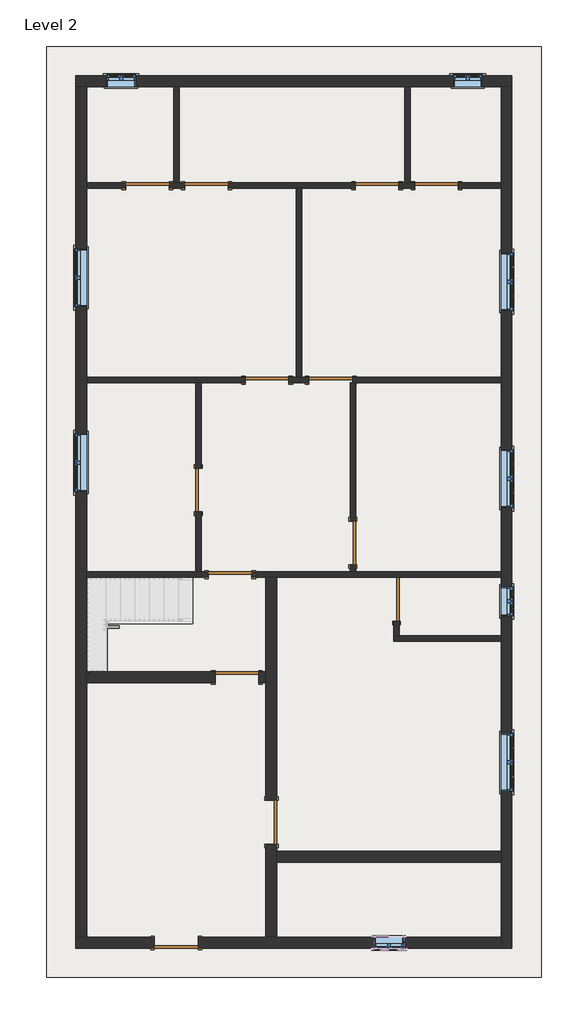
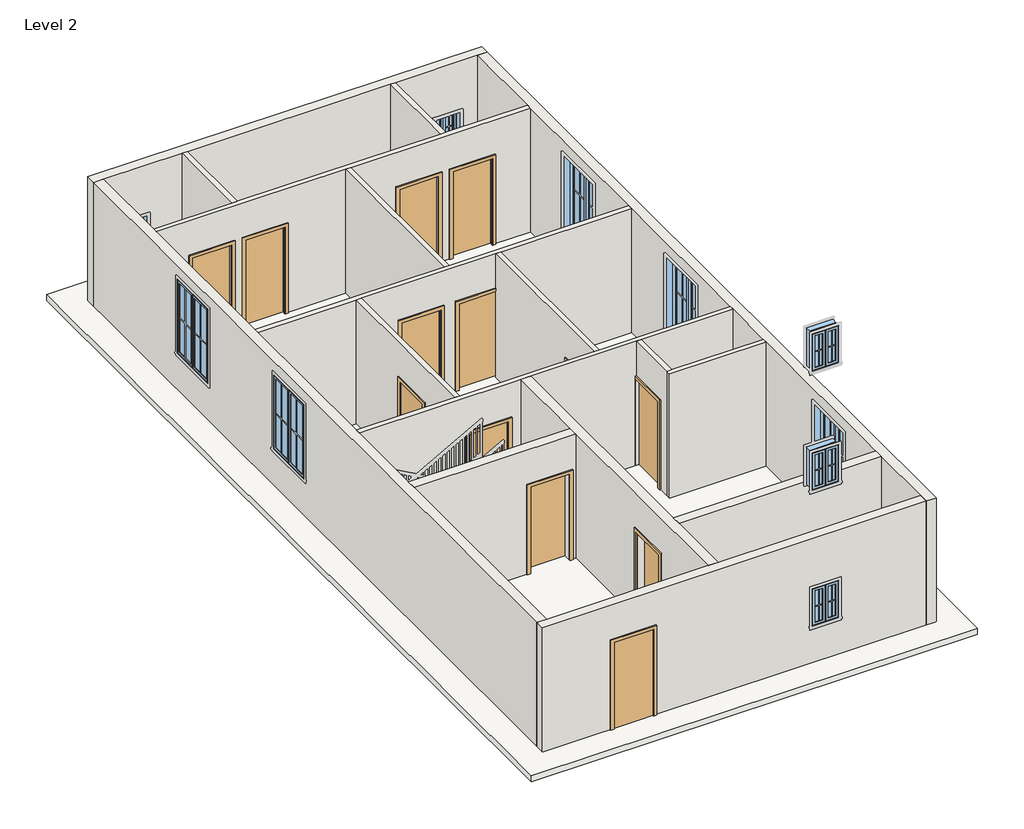
# One storey, part 1 of 3: 17 walls, 13 doors, 11 windows, 1 slab.
"""IFC4 building model written with IfcOpenShell, lengths in millimetres."""

from ifc_helpers import new_model, si_unit, frame, origin, place, context, project, spatial, polyline, outline, extrude, faceted_brep, transform, mapped, element, save
from components import door_305aa2a5, door_e5f9f3c4, door_0ca8825f, window_c417fced, window_6ca1769e

model = new_model("IFC4")

# Units and contexts
model_context = context("Model", 3, world=origin())
ifc_project = project(units=[si_unit("LENGTHUNIT", "METRE", prefix="MILLI")], contexts=[model_context])

# Site, building, storey
site = spatial("IfcSite", under=ifc_project)
building = spatial("IfcBuilding", under=site)
storey = spatial("IfcBuildingStorey", under=building, Name="Level 2", Elevation=3048.0)

# Doors
placement = place(None, origin())
door_shape = door_305aa2a5(model_context)
element("IfcDoor", 1, ObjectType="Single-Flush : 36\" x 84\"", at=placement, inside=storey, context=model_context, shape_type="MappedRepresentation", body=[
    mapped(door_shape, transform((4013.2, 11918.95, 3048.0), x_axis=(-1.0, 0.0, 0.0), y_axis=(0.0, -1.0, 0.0), z_axis=(0.0, 0.0, 1.0))),
])
element("IfcDoor", 2, ObjectType="Single-Flush : 36\" x 84\"", at=placement, inside=storey, context=model_context, shape_type="MappedRepresentation", body=[
    mapped(door_shape, transform((8832.85, 11918.95, 3048.0), x_axis=(-1.0, 0.0, 0.0), y_axis=(0.0, -1.0, 0.0), z_axis=(0.0, 0.0, 1.0))),
])
element("IfcDoor", 3, ObjectType="Single-Flush : 36\" x 84\"", at=placement, inside=storey, context=model_context, shape_type="MappedRepresentation", body=[
    mapped(door_shape, transform((6616.7, 7842.25, 3048.0), x_axis=(-1.0, 0.0, 0.0), y_axis=(0.0, -1.0, 0.0), z_axis=(0.0, 0.0, 1.0))),
])
element("IfcDoor", 4, ObjectType="Single-Flush : 36\" x 84\"", at=placement, inside=storey, context=model_context, shape_type="MappedRepresentation", body=[
    mapped(door_shape, transform((3841.75, 5537.2, 3048.0), x_axis=(0.0, -1.0, 0.0), y_axis=(1.0, 0.0, 0.0), z_axis=(0.0, 0.0, 1.0))),
])
door_2_shape = door_e5f9f3c4(model_context)
element("IfcDoor", 5, ObjectType="Single-Flush : 36\" x 84\"", at=placement, inside=storey, context=model_context, shape_type="MappedRepresentation", body=[
    mapped(door_2_shape, transform((2774.95, 11918.95, 3048.0), x_axis=(1.0, 0.0, 0.0), y_axis=(0.0, 1.0, 0.0), z_axis=(0.0, 0.0, 1.0))),
])
element("IfcDoor", 6, ObjectType="Single-Flush : 36\" x 84\"", at=placement, inside=storey, context=model_context, shape_type="MappedRepresentation", body=[
    mapped(door_2_shape, transform((7588.25, 11918.95, 3048.0), x_axis=(1.0, 0.0, 0.0), y_axis=(0.0, 1.0, 0.0), z_axis=(0.0, 0.0, 1.0))),
])
element("IfcDoor", 7, ObjectType="Single-Flush : 36\" x 84\"", at=placement, inside=storey, context=model_context, shape_type="MappedRepresentation", body=[
    mapped(door_2_shape, transform((5283.2, 7842.25, 3048.0), x_axis=(1.0, 0.0, 0.0), y_axis=(0.0, 1.0, 0.0), z_axis=(0.0, 0.0, 1.0))),
])
element("IfcDoor", 8, ObjectType="Single-Flush : 36\" x 84\"", at=placement, inside=storey, context=model_context, shape_type="MappedRepresentation", body=[
    mapped(door_2_shape, transform((4508.5, 3765.55, 3048.0), x_axis=(1.0, 0.0, 0.0), y_axis=(0.0, 1.0, 0.0), z_axis=(0.0, 0.0, 1.0))),
])
element("IfcDoor", 9, ObjectType="Single-Flush : 36\" x 84\"", at=placement, inside=storey, context=model_context, shape_type="MappedRepresentation", body=[
    mapped(door_2_shape, transform((7080.25, 4432.3, 3048.0), x_axis=(0.0, -1.0, 0.0), y_axis=(1.0, 0.0, 0.0), z_axis=(0.0, 0.0, 1.0))),
])
element("IfcDoor", 10, ObjectType="Single-Flush : 36\" x 84\"", at=placement, inside=storey, context=model_context, shape_type="MappedRepresentation", body=[
    mapped(door_2_shape, transform((7994.65, 3251.2, 3048.0), x_axis=(0.0, -1.0, 0.0), y_axis=(1.0, 0.0, 0.0), z_axis=(0.0, 0.0, 1.0))),
])
door_3_shape = door_0ca8825f(model_context)
element("IfcDoor", 11, ObjectType="Single-Flush : 36\" x 84\"", at=placement, inside=storey, context=model_context, shape_type="MappedRepresentation", body=[
    mapped(door_3_shape, transform((4648.2, 1612.9, 3048.0), x_axis=(1.0, 0.0, 0.0), y_axis=(0.0, 1.0, 0.0), z_axis=(0.0, 0.0, 1.0))),
])
element("IfcDoor", 12, ObjectType="Single-Flush : 36\" x 84\"", at=placement, inside=storey, context=model_context, shape_type="MappedRepresentation", body=[
    mapped(door_3_shape, transform((5372.1, -1422.4, 3048.0), x_axis=(0.0, -1.0, 0.0), y_axis=(1.0, 0.0, 0.0), z_axis=(0.0, 0.0, 1.0))),
])
element("IfcDoor", 13, ObjectType="Single-Flush : 36\" x 84\"", at=placement, inside=storey, context=model_context, shape_type="MappedRepresentation", body=[
    mapped(door_3_shape, transform((3378.2, -3949.7, 3048.0), x_axis=(-1.0, 0.0, 0.0), y_axis=(0.0, -1.0, 0.0), z_axis=(0.0, 0.0, 1.0))),
])

# Slab
element("IfcSlab", 14, ObjectType="Generic - 12\"", at=placement, inside=storey, context=model_context, shape_type="SweptSolid", body=[
    extrude(outline(polyline([(11023.6, 14833.6), (11023.6, -4673.6), (660.4, -4673.6), (660.4, 14833.6), (11023.6, 14833.6)])), frame((0.0, 0.0, 2895.6), z_axis=(0.0, 0.0, 1.0), x_axis=(1.0, 0.0, 0.0)), (0.0, 0.0, 1.0), 152.4),
])

# Walls
element("IfcWall", 15, ObjectType="Generic - 5\"", at=placement, inside=storey, context=model_context, shape_type="Brep", body=[
    faceted_brep([(8045.45, 11861.8, 3048.0), (8375.65, 11861.8, 3048.0), (8375.65, 11861.8, 5181.6), (9290.05, 11861.8, 5181.6), (9290.05, 11861.8, 3048.0), (10185.4, 11861.8, 3048.0), (10185.4, 11861.8, 6096.0), (6007.1, 11861.8, 6096.0), (5892.8, 11861.8, 6096.0), (1498.6, 11861.8, 6096.0), (1498.6, 11861.8, 3048.0), (2317.75, 11861.8, 3048.0), (2317.75, 11861.8, 5181.6), (3232.15, 11861.8, 5181.6), (3232.15, 11861.8, 3048.0), (3556.0, 11861.8, 3048.0), (3556.0, 11861.8, 5181.6), (4470.4, 11861.8, 5181.6), (4470.4, 11861.8, 3048.0), (5892.8, 11861.8, 3048.0), (6007.1, 11861.8, 3048.0), (7131.05, 11861.8, 3048.0), (7131.05, 11861.8, 5181.6), (8045.45, 11861.8, 5181.6), (8375.65, 11976.1, 5181.6), (8375.65, 11976.1, 3048.0), (8280.4, 11976.1, 3048.0), (8166.1, 11976.1, 3048.0), (8045.45, 11976.1, 3048.0), (8045.45, 11976.1, 5181.6), (7131.05, 11976.1, 5181.6), (7131.05, 11976.1, 3048.0), (4470.4, 11976.1, 3048.0), (4470.4, 11976.1, 5181.6), (3556.0, 11976.1, 5181.6), (3556.0, 11976.1, 3048.0), (3441.7, 11976.1, 3048.0), (3327.4, 11976.1, 3048.0), (3232.15, 11976.1, 3048.0), (3232.15, 11976.1, 5181.6), (2317.75, 11976.1, 5181.6), (2317.75, 11976.1, 3048.0), (1498.6, 11976.1, 3048.0), (1498.6, 11976.1, 6096.0), (3327.4, 11976.1, 6096.0), (3441.7, 11976.1, 6096.0), (8166.1, 11976.1, 6096.0), (8280.4, 11976.1, 6096.0), (10185.4, 11976.1, 6096.0), (10185.4, 11976.1, 3048.0), (9290.05, 11976.1, 3048.0), (9290.05, 11976.1, 5181.6)], [[[0, 1, 2, 3, 4, 5, 6, 7, 8, 9, 10, 11, 12, 13, 14, 15, 16, 17, 18, 19, 20, 21, 22, 23]], [[24, 25, 26, 27, 28, 29, 30, 31, 32, 33, 34, 35, 36, 37, 38, 39, 40, 41, 42, 43, 44, 45, 46, 47, 48, 49, 50, 51]], [[11, 10, 42, 41]], [[15, 14, 38, 37, 36, 35]], [[21, 20, 19, 18, 32, 31]], [[50, 49, 5, 4]], [[28, 27, 26, 25, 1, 0]], [[9, 8, 7, 6, 48, 47, 46, 45, 44, 43]], [[6, 5, 49, 48]], [[10, 9, 43, 42]], [[16, 15, 35, 34]], [[17, 16, 34, 33]], [[18, 17, 33, 32]], [[39, 38, 14, 13]], [[40, 39, 13, 12]], [[41, 40, 12, 11]], [[29, 28, 0, 23]], [[30, 29, 23, 22]], [[31, 30, 22, 21]], [[2, 1, 25, 24]], [[3, 2, 24, 51]], [[4, 3, 51, 50]]]),
])
element("IfcWall", 16, ObjectType="Generic - 5\"", at=placement, inside=storey, context=model_context, shape_type="Brep", body=[
    faceted_brep([(5740.4, 7785.1, 3048.0), (6159.5, 7785.1, 3048.0), (6159.5, 7785.1, 5181.6), (7073.9, 7785.1, 5181.6), (7073.9, 7785.1, 3048.0), (7137.4, 7785.1, 3048.0), (10185.4, 7785.1, 3048.0), (10185.4, 7785.1, 6096.0), (7137.4, 7785.1, 6096.0), (7023.1, 7785.1, 6096.0), (3898.9, 7785.1, 6096.0), (3784.6, 7785.1, 6096.0), (1498.6, 7785.1, 6096.0), (1498.6, 7785.1, 3048.0), (3784.6, 7785.1, 3048.0), (3898.9, 7785.1, 3048.0), (4826.0, 7785.1, 3048.0), (4826.0, 7785.1, 5181.6), (5740.4, 7785.1, 5181.6), (6159.5, 7899.4, 5181.6), (6159.5, 7899.4, 3048.0), (6007.1, 7899.4, 3048.0), (5892.8, 7899.4, 3048.0), (5740.4, 7899.4, 3048.0), (5740.4, 7899.4, 5181.6), (4826.0, 7899.4, 5181.6), (4826.0, 7899.4, 3048.0), (1498.6, 7899.4, 3048.0), (1498.6, 7899.4, 6096.0), (5892.8, 7899.4, 6096.0), (6007.1, 7899.4, 6096.0), (10185.4, 7899.4, 6096.0), (10185.4, 7899.4, 3048.0), (7073.9, 7899.4, 3048.0), (7073.9, 7899.4, 5181.6)], [[[0, 1, 2, 3, 4, 5, 6, 7, 8, 9, 10, 11, 12, 13, 14, 15, 16, 17, 18]], [[19, 20, 21, 22, 23, 24, 25, 26, 27, 28, 29, 30, 31, 32, 33, 34]], [[16, 15, 14, 13, 27, 26]], [[33, 32, 6, 5, 4]], [[23, 22, 21, 20, 1, 0]], [[12, 11, 10, 9, 8, 7, 31, 30, 29, 28]], [[7, 6, 32, 31]], [[13, 12, 28, 27]], [[24, 23, 0, 18]], [[25, 24, 18, 17]], [[26, 25, 17, 16]], [[2, 1, 20, 19]], [[3, 2, 19, 34]], [[4, 3, 34, 33]]]),
])
element("IfcWall", 17, ObjectType="Generic - 5\"", at=placement, inside=storey, context=model_context, shape_type="SweptSolid", body=[
    extrude(outline(polyline([(5080.0, 5181.6), (5080.0, 3048.0), (3822.7, 3048.0), (3822.7, 6096.0), (7785.1, 6096.0), (7785.1, 3048.0), (5994.4, 3048.0), (5994.4, 5181.6), (5080.0, 5181.6)])), frame((3784.6, 0.0, 0.0), z_axis=(1.0, 0.0, 0.0), x_axis=(0.0, 1.0, 0.0)), (0.0, 0.0, 1.0), 114.3),
])
element("IfcWall", 18, ObjectType="Generic - 5\"", at=placement, inside=storey, context=model_context, shape_type="Brep", body=[
    faceted_brep([(4965.7, 3708.4, 5181.6), (4965.7, 3708.4, 3048.0), (5257.8, 3708.4, 3048.0), (5486.4, 3708.4, 3048.0), (10185.4, 3708.4, 3048.0), (10185.4, 3708.4, 6096.0), (8051.8, 3708.4, 6096.0), (7937.5, 3708.4, 6096.0), (5486.4, 3708.4, 6096.0), (5257.8, 3708.4, 6096.0), (1498.6, 3708.4, 6096.0), (1498.6, 3708.4, 3048.0), (4051.3, 3708.4, 3048.0), (4051.3, 3708.4, 5181.6), (10185.4, 3822.7, 3048.0), (7137.4, 3822.7, 3048.0), (7023.1, 3822.7, 3048.0), (4965.7, 3822.7, 3048.0), (4965.7, 3822.7, 5181.6), (4051.3, 3822.7, 5181.6), (4051.3, 3822.7, 3048.0), (3898.9, 3822.7, 3048.0), (3784.6, 3822.7, 3048.0), (1498.6, 3822.7, 3048.0), (1498.6, 3822.7, 6096.0), (3784.6, 3822.7, 6096.0), (3898.9, 3822.7, 6096.0), (7023.1, 3822.7, 6096.0), (7137.4, 3822.7, 6096.0), (10185.4, 3822.7, 6096.0)], [[[0, 1, 2, 3, 4, 5, 6, 7, 8, 9, 10, 11, 12, 13]], [[14, 15, 16, 17, 18, 19, 20, 21, 22, 23, 24, 25, 26, 27, 28, 29]], [[12, 11, 23, 22, 21, 20]], [[4, 3, 2, 1, 17, 16, 15, 14]], [[10, 9, 8, 7, 6, 5, 29, 28, 27, 26, 25, 24]], [[5, 4, 14, 29]], [[11, 10, 24, 23]], [[18, 17, 1, 0]], [[19, 18, 0, 13]], [[20, 19, 13, 12]]]),
])
element("IfcWall", 19, ObjectType="Generic - 5\"", at=placement, inside=storey, context=model_context, shape_type="Brep", body=[
    faceted_brep([(10185.4, 2489.2, 3048.0), (8051.8, 2489.2, 3048.0), (7937.5, 2489.2, 3048.0), (7937.5, 2489.2, 6096.0), (8051.8, 2489.2, 6096.0), (10185.4, 2489.2, 6096.0), (10185.4, 2374.9, 3048.0), (10185.4, 2374.9, 6096.0), (7937.5, 2374.9, 6096.0), (7937.5, 2374.9, 3048.0)], [[[0, 1, 2, 3, 4, 5]], [[6, 7, 8, 9]], [[2, 1, 0, 6, 9]], [[5, 4, 3, 8, 7]], [[0, 5, 7, 6]], [[3, 2, 9, 8]]]),
])
element("IfcWall", 20, ObjectType="Generic - 5\"", at=placement, inside=storey, context=model_context, shape_type="SweptSolid", body=[
    extrude(outline(polyline([(2489.2, 6096.0), (3708.4, 6096.0), (3708.4, 5181.6), (2794.0, 5181.6), (2794.0, 3048.0), (2489.2, 3048.0), (2489.2, 6096.0)])), frame((7937.5, 0.0, 0.0), z_axis=(1.0, 0.0, 0.0), x_axis=(0.0, 1.0, 0.0)), (0.0, 0.0, 1.0), 114.3),
])
element("IfcWall", 21, ObjectType="Generic - 5\"", at=placement, inside=storey, context=model_context, shape_type="Brep", body=[
    faceted_brep([(7023.1, 3975.1, 5181.6), (7023.1, 3975.1, 3048.0), (7023.1, 3822.7, 3048.0), (7023.1, 3822.7, 6096.0), (7023.1, 7785.1, 6096.0), (7023.1, 7785.1, 3048.0), (7023.1, 4889.5, 3048.0), (7023.1, 4889.5, 5181.6), (7137.4, 3822.7, 3048.0), (7137.4, 3975.1, 3048.0), (7137.4, 3975.1, 5181.6), (7137.4, 4889.5, 5181.6), (7137.4, 4889.5, 3048.0), (7137.4, 7785.1, 3048.0), (7137.4, 7785.1, 6096.0), (7137.4, 3822.7, 6096.0), (7073.9, 7785.1, 3048.0)], [[[0, 1, 2, 3, 4, 5, 6, 7]], [[8, 9, 10, 11, 12, 13, 14, 15]], [[6, 5, 16, 13, 12]], [[2, 1, 9, 8]], [[4, 3, 15, 14]], [[5, 4, 14, 13, 16]], [[3, 2, 8, 15]], [[10, 9, 1, 0]], [[11, 10, 0, 7]], [[12, 11, 7, 6]]]),
])
element("IfcWall", 22, ObjectType="Generic - 5\"", at=placement, inside=storey, context=model_context, shape_type="SweptSolid", body=[
    extrude(outline(polyline([(3327.4, 11976.1), (3327.4, 13995.4), (3441.7, 13995.4), (3441.7, 11976.1), (3327.4, 11976.1)])), frame((0.0, 0.0, 3048.0), z_axis=(0.0, 0.0, 1.0), x_axis=(1.0, 0.0, 0.0)), (0.0, 0.0, 1.0), 3048.0),
])
element("IfcWall", 23, ObjectType="Generic - 5\"", at=placement, inside=storey, context=model_context, shape_type="SweptSolid", body=[
    extrude(outline(polyline([(8166.1, 11976.1), (8166.1, 13995.4), (8280.4, 13995.4), (8280.4, 11976.1), (8166.1, 11976.1)])), frame((0.0, 0.0, 3048.0), z_axis=(0.0, 0.0, 1.0), x_axis=(1.0, 0.0, 0.0)), (0.0, 0.0, 1.0), 3048.0),
])
element("IfcWall", 24, ObjectType="Generic - 5\"", at=placement, inside=storey, context=model_context, shape_type="SweptSolid", body=[
    extrude(outline(polyline([(5892.8, 7899.4), (5892.8, 11861.8), (6007.1, 11861.8), (6007.1, 7899.4), (5892.8, 7899.4)])), frame((0.0, 0.0, 3048.0), z_axis=(0.0, 0.0, 1.0), x_axis=(1.0, 0.0, 0.0)), (0.0, 0.0, 1.0), 3048.0),
])
element("IfcWall", 25, ObjectType="Generic - 8\"", at=placement, inside=storey, context=model_context, shape_type="Brep", body=[
    faceted_brep([(1270.0, 13995.4, 3048.0), (1498.6, 13995.4, 3048.0), (3327.4, 13995.4, 3048.0), (3441.7, 13995.4, 3048.0), (8166.1, 13995.4, 3048.0), (8280.4, 13995.4, 3048.0), (10185.4, 13995.4, 3048.0), (10414.0, 13995.4, 3048.0), (10414.0, 13995.4, 6096.0), (10185.4, 13995.4, 6096.0), (8280.4, 13995.4, 6096.0), (8166.1, 13995.4, 6096.0), (3441.7, 13995.4, 6096.0), (3327.4, 13995.4, 6096.0), (1498.6, 13995.4, 6096.0), (1270.0, 13995.4, 6096.0), (9791.7, 13995.4, 4876.8), (9791.7, 13995.4, 3962.4), (9182.1, 13995.4, 3962.4), (9182.1, 13995.4, 4876.8), (2527.3, 13995.4, 4876.8), (2527.3, 13995.4, 3962.4), (1917.7, 13995.4, 3962.4), (1917.7, 13995.4, 4876.8), (1270.0, 14224.0, 3048.0), (1270.0, 14224.0, 6096.0), (10414.0, 14224.0, 6096.0), (10414.0, 14224.0, 3048.0), (9791.7, 14224.0, 4876.8), (9182.1, 14224.0, 4876.8), (9182.1, 14224.0, 3962.4), (9791.7, 14224.0, 3962.4), (2527.3, 14224.0, 4876.8), (1917.7, 14224.0, 4876.8), (1917.7, 14224.0, 3962.4), (2527.3, 14224.0, 3962.4)], [[[0, 1, 2, 3, 4, 5, 6, 7, 8, 9, 10, 11, 12, 13, 14, 15], [16, 17, 18, 19], [20, 21, 22, 23]], [[24, 25, 26, 27], [28, 29, 30, 31], [32, 33, 34, 35]], [[7, 6, 5, 4, 3, 2, 1, 0, 24, 27]], [[15, 14, 13, 12, 11, 10, 9, 8, 26, 25]], [[8, 7, 27, 26]], [[0, 15, 25, 24]], [[17, 16, 28, 31]], [[18, 17, 31, 30]], [[19, 18, 30, 29]], [[16, 19, 29, 28]], [[21, 20, 32, 35]], [[22, 21, 35, 34]], [[23, 22, 34, 33]], [[20, 23, 33, 32]]]),
])
element("IfcWall", 26, ObjectType="Generic - 8\"", at=placement, inside=storey, context=model_context, shape_type="Brep", body=[
    faceted_brep([(10185.4, 13995.4, 3048.0), (10185.4, 11976.1, 3048.0), (10185.4, 11861.8, 3048.0), (10185.4, 7899.4, 3048.0), (10185.4, 7785.1, 3048.0), (10185.4, 3822.7, 3048.0), (10185.4, 3708.4, 3048.0), (10185.4, 2489.2, 3048.0), (10185.4, 2374.9, 3048.0), (10185.4, -2032.0, 3048.0), (10185.4, -2260.6, 3048.0), (10185.4, -3835.4, 3048.0), (10185.4, -4064.0, 3048.0), (10185.4, -4064.0, 6096.0), (10185.4, -3835.4, 6096.0), (10185.4, -2260.6, 6096.0), (10185.4, -2032.0, 6096.0), (10185.4, 2374.9, 6096.0), (10185.4, 2489.2, 6096.0), (10185.4, 3708.4, 6096.0), (10185.4, 3822.7, 6096.0), (10185.4, 7785.1, 6096.0), (10185.4, 7899.4, 6096.0), (10185.4, 11861.8, 6096.0), (10185.4, 11976.1, 6096.0), (10185.4, 13995.4, 6096.0), (10185.4, 9296.4, 5791.2), (10185.4, 9296.4, 3962.4), (10185.4, 10515.6, 3962.4), (10185.4, 10515.6, 5791.2), (10185.4, 5168.9, 5791.2), (10185.4, 5168.9, 3962.4), (10185.4, 6388.1, 3962.4), (10185.4, 6388.1, 5791.2), (10185.4, -774.7, 5791.2), (10185.4, -774.7, 3962.4), (10185.4, 444.5, 3962.4), (10185.4, 444.5, 5791.2), (10185.4, 2901.95, 4876.8), (10185.4, 2901.95, 3962.4), (10185.4, 3511.55, 3962.4), (10185.4, 3511.55, 4876.8), (10414.0, 13995.4, 3048.0), (10414.0, 13995.4, 6096.0), (10414.0, -4064.0, 6096.0), (10414.0, -4064.0, 3048.0), (10414.0, 9296.4, 5791.2), (10414.0, 10515.6, 5791.2), (10414.0, 10515.6, 3962.4), (10414.0, 9296.4, 3962.4), (10414.0, 5168.9, 5791.2), (10414.0, 6388.1, 5791.2), (10414.0, 6388.1, 3962.4), (10414.0, 5168.9, 3962.4), (10414.0, -774.7, 5791.2), (10414.0, 444.5, 5791.2), (10414.0, 444.5, 3962.4), (10414.0, -774.7, 3962.4), (10414.0, 2901.95, 4876.8), (10414.0, 3511.55, 4876.8), (10414.0, 3511.55, 3962.4), (10414.0, 2901.95, 3962.4)], [[[0, 1, 2, 3, 4, 5, 6, 7, 8, 9, 10, 11, 12, 13, 14, 15, 16, 17, 18, 19, 20, 21, 22, 23, 24, 25], [26, 27, 28, 29], [30, 31, 32, 33], [34, 35, 36, 37], [38, 39, 40, 41]], [[42, 43, 44, 45], [46, 47, 48, 49], [50, 51, 52, 53], [54, 55, 56, 57], [58, 59, 60, 61]], [[12, 11, 10, 9, 8, 7, 6, 5, 4, 3, 2, 1, 0, 42, 45]], [[25, 24, 23, 22, 21, 20, 19, 18, 17, 16, 15, 14, 13, 44, 43]], [[0, 25, 43, 42]], [[13, 12, 45, 44]], [[27, 26, 46, 49]], [[28, 27, 49, 48]], [[29, 28, 48, 47]], [[26, 29, 47, 46]], [[31, 30, 50, 53]], [[32, 31, 53, 52]], [[33, 32, 52, 51]], [[30, 33, 51, 50]], [[35, 34, 54, 57]], [[36, 35, 57, 56]], [[37, 36, 56, 55]], [[34, 37, 55, 54]], [[39, 38, 58, 61]], [[40, 39, 61, 60]], [[41, 40, 60, 59]], [[38, 41, 59, 58]]]),
])
element("IfcWall", 27, ObjectType="Generic - 8\"", at=placement, inside=storey, context=model_context, shape_type="Brep", body=[
    faceted_brep([(2921.0, -3835.4, 5181.6), (2921.0, -3835.4, 3048.0), (1498.6, -3835.4, 3048.0), (1270.0, -3835.4, 3048.0), (1270.0, -3835.4, 6096.0), (1498.6, -3835.4, 6096.0), (5257.8, -3835.4, 6096.0), (5486.4, -3835.4, 6096.0), (10185.4, -3835.4, 6096.0), (10185.4, -3835.4, 3048.0), (5486.4, -3835.4, 3048.0), (5257.8, -3835.4, 3048.0), (3835.4, -3835.4, 3048.0), (3835.4, -3835.4, 5181.6), (7531.1, -3835.4, 4876.8), (7531.1, -3835.4, 3962.4), (8140.7, -3835.4, 3962.4), (8140.7, -3835.4, 4876.8), (1270.0, -4064.0, 3048.0), (2921.0, -4064.0, 3048.0), (2921.0, -4064.0, 5181.6), (3835.4, -4064.0, 5181.6), (3835.4, -4064.0, 3048.0), (10185.4, -4064.0, 3048.0), (10185.4, -4064.0, 6096.0), (1270.0, -4064.0, 6096.0), (7531.1, -4064.0, 4876.8), (8140.7, -4064.0, 4876.8), (8140.7, -4064.0, 3962.4), (7531.1, -4064.0, 3962.4)], [[[0, 1, 2, 3, 4, 5, 6, 7, 8, 9, 10, 11, 12, 13], [14, 15, 16, 17]], [[18, 19, 20, 21, 22, 23, 24, 25], [26, 27, 28, 29]], [[3, 2, 1, 19, 18]], [[12, 11, 10, 9, 23, 22]], [[8, 7, 6, 5, 4, 25, 24]], [[9, 8, 24, 23]], [[4, 3, 18, 25]], [[20, 19, 1, 0]], [[21, 20, 0, 13]], [[22, 21, 13, 12]], [[15, 14, 26, 29]], [[16, 15, 29, 28]], [[17, 16, 28, 27]], [[14, 17, 27, 26]]]),
])
element("IfcWall", 28, ObjectType="Generic - 8\"", at=placement, inside=storey, context=model_context, shape_type="Brep", body=[
    faceted_brep([(1498.6, -3835.4, 3048.0), (1498.6, 1498.6, 3048.0), (1498.6, 1727.2, 3048.0), (1498.6, 3708.4, 3048.0), (1498.6, 3822.7, 3048.0), (1498.6, 7785.1, 3048.0), (1498.6, 7899.4, 3048.0), (1498.6, 11861.8, 3048.0), (1498.6, 11976.1, 3048.0), (1498.6, 13995.4, 3048.0), (1498.6, 13995.4, 6096.0), (1498.6, 11976.1, 6096.0), (1498.6, 11861.8, 6096.0), (1498.6, 7899.4, 6096.0), (1498.6, 7785.1, 6096.0), (1498.6, 3822.7, 6096.0), (1498.6, 3708.4, 6096.0), (1498.6, 1727.2, 6096.0), (1498.6, 1498.6, 6096.0), (1498.6, -3835.4, 6096.0), (1498.6, 6724.65, 5791.2), (1498.6, 6724.65, 3962.4), (1498.6, 5505.45, 3962.4), (1498.6, 5505.45, 5791.2), (1498.6, 10598.15, 5791.2), (1498.6, 10598.15, 3962.4), (1498.6, 9378.95, 3962.4), (1498.6, 9378.95, 5791.2), (1270.0, -3835.4, 3048.0), (1270.0, -3835.4, 6096.0), (1270.0, 13995.4, 6096.0), (1270.0, 13995.4, 3048.0), (1270.0, 6724.65, 5791.2), (1270.0, 5505.45, 5791.2), (1270.0, 5505.45, 3962.4), (1270.0, 6724.65, 3962.4), (1270.0, 10598.15, 5791.2), (1270.0, 9378.95, 5791.2), (1270.0, 9378.95, 3962.4), (1270.0, 10598.15, 3962.4)], [[[0, 1, 2, 3, 4, 5, 6, 7, 8, 9, 10, 11, 12, 13, 14, 15, 16, 17, 18, 19], [20, 21, 22, 23], [24, 25, 26, 27]], [[28, 29, 30, 31], [32, 33, 34, 35], [36, 37, 38, 39]], [[9, 8, 7, 6, 5, 4, 3, 2, 1, 0, 28, 31]], [[19, 18, 17, 16, 15, 14, 13, 12, 11, 10, 30, 29]], [[10, 9, 31, 30]], [[21, 20, 32, 35]], [[22, 21, 35, 34]], [[23, 22, 34, 33]], [[20, 23, 33, 32]], [[25, 24, 36, 39]], [[26, 25, 39, 38]], [[27, 26, 38, 37]], [[24, 27, 37, 36]], [[0, 19, 29, 28]]]),
])
element("IfcWall", 29, ObjectType="Generic - 8\"", at=placement, inside=storey, context=model_context, shape_type="SweptSolid", body=[
    extrude(outline(polyline([(5181.6, 5105.4), (3048.0, 5105.4), (3048.0, 5257.8), (6096.0, 5257.8), (6096.0, 1498.6), (3048.0, 1498.6), (3048.0, 4191.0), (5181.6, 4191.0), (5181.6, 5105.4)])), frame((0.0, 1498.6, 0.0), z_axis=(0.0, 1.0, 0.0), x_axis=(0.0, 0.0, 1.0)), (0.0, 0.0, 1.0), 228.6),
])
element("IfcWall", 30, ObjectType="Generic - 8\"", at=placement, inside=storey, context=model_context, shape_type="Brep", body=[
    faceted_brep([(5257.8, -1879.6, 5181.6), (5257.8, -1879.6, 3048.0), (5257.8, -3835.4, 3048.0), (5257.8, -3835.4, 6096.0), (5257.8, 1498.6, 6096.0), (5257.8, 1727.2, 6096.0), (5257.8, 3708.4, 6096.0), (5257.8, 3708.4, 3048.0), (5257.8, 1727.2, 3048.0), (5257.8, 1498.6, 3048.0), (5257.8, -965.2, 3048.0), (5257.8, -965.2, 5181.6), (5486.4, -3835.4, 3048.0), (5486.4, -2260.6, 3048.0), (5486.4, -2032.0, 3048.0), (5486.4, -1879.6, 3048.0), (5486.4, -1879.6, 5181.6), (5486.4, -965.2, 5181.6), (5486.4, -965.2, 3048.0), (5486.4, 3708.4, 3048.0), (5486.4, 3708.4, 6096.0), (5486.4, -2032.0, 6096.0), (5486.4, -2260.6, 6096.0), (5486.4, -3835.4, 6096.0)], [[[0, 1, 2, 3, 4, 5, 6, 7, 8, 9, 10, 11]], [[12, 13, 14, 15, 16, 17, 18, 19, 20, 21, 22, 23]], [[2, 1, 15, 14, 13, 12]], [[10, 9, 8, 7, 19, 18]], [[6, 5, 4, 3, 23, 22, 21, 20]], [[3, 2, 12, 23]], [[7, 6, 20, 19]], [[16, 15, 1, 0]], [[17, 16, 0, 11]], [[18, 17, 11, 10]]]),
])
element("IfcWall", 31, ObjectType="Generic - 8\"", at=placement, inside=storey, context=model_context, shape_type="SweptSolid", body=[
    extrude(outline(polyline([(10185.4, -2260.6), (5486.4, -2260.6), (5486.4, -2032.0), (10185.4, -2032.0), (10185.4, -2260.6)])), frame((0.0, 0.0, 3048.0), z_axis=(0.0, 0.0, 1.0), x_axis=(1.0, 0.0, 0.0)), (0.0, 0.0, 1.0), 3048.0),
])

# Windows
window_shape = window_c417fced(model_context)
element("IfcWindow", 32, ObjectType="Window-Casement-Double : 24\" x 36\"", at=placement, inside=storey, context=model_context, shape_type="MappedRepresentation", body=[
    mapped(window_shape, transform((10299.7, 3206.75, 3048.0), x_axis=(0.0, -1.0, 0.0), y_axis=(1.0, 0.0, 0.0), z_axis=(0.0, 0.0, 1.0))),
])
element("IfcWindow", 33, ObjectType="Window-Casement-Double : 24\" x 36\"", at=placement, inside=storey, context=model_context, shape_type="MappedRepresentation", body=[
    mapped(window_shape, transform((9486.9, 14109.7, 3048.0), x_axis=(1.0, 0.0, 0.0), y_axis=(0.0, 1.0, 0.0), z_axis=(0.0, 0.0, 1.0))),
])
element("IfcWindow", 34, ObjectType="Window-Casement-Double : 24\" x 36\"", at=placement, inside=storey, context=model_context, shape_type="MappedRepresentation", body=[
    mapped(window_shape, transform((2222.5, 14109.7, 3048.0), x_axis=(1.0, 0.0, 0.0), y_axis=(0.0, 1.0, 0.0), z_axis=(0.0, 0.0, 1.0))),
])
element("IfcWindow", 35, ObjectType="Window-Casement-Double : 24\" x 36\"", at=placement, inside=storey, context=model_context, shape_type="MappedRepresentation", body=[
    mapped(window_shape, transform((7835.9, -3949.7, 3048.0), x_axis=(-1.0, 0.0, 0.0), y_axis=(0.0, -1.0, 0.0), z_axis=(0.0, 0.0, 1.0))),
])
element("IfcWindow", 36, ObjectType="Window-Casement-Double : 24\" x 36\"", at=placement, inside=storey, context=model_context, shape_type="MappedRepresentation", body=[
    mapped(window_shape, transform((7835.9, -3949.7, 6386.4257161), x_axis=(-1.0, 0.0, 0.0), y_axis=(0.0, -1.0, 0.0), z_axis=(0.0, 0.0, 1.0))),
])
element("IfcWindow", 37, ObjectType="Window-Casement-Double : 24\" x 36\"", at=placement, inside=storey, context=model_context, shape_type="MappedRepresentation", body=[
    mapped(window_shape, transform((7835.9, -3949.7, 9310.6873604), x_axis=(-1.0, 0.0, 0.0), y_axis=(0.0, -1.0, 0.0), z_axis=(0.0, 0.0, 1.0))),
])
window_2_shape = window_6ca1769e(model_context)
element("IfcWindow", 38, ObjectType="Window-Casement-Double : 48\" x 72\"", at=placement, inside=storey, context=model_context, shape_type="MappedRepresentation", body=[
    mapped(window_2_shape, transform((1384.3, 6115.05, 3048.0), x_axis=(0.0, 1.0, 0.0), y_axis=(-1.0, 0.0, 0.0), z_axis=(0.0, 0.0, 1.0))),
])
element("IfcWindow", 39, ObjectType="Window-Casement-Double : 48\" x 72\"", at=placement, inside=storey, context=model_context, shape_type="MappedRepresentation", body=[
    mapped(window_2_shape, transform((1384.3, 9988.55, 3048.0), x_axis=(0.0, 1.0, 0.0), y_axis=(-1.0, 0.0, 0.0), z_axis=(0.0, 0.0, 1.0))),
])
element("IfcWindow", 40, ObjectType="Window-Casement-Double : 48\" x 72\"", at=placement, inside=storey, context=model_context, shape_type="MappedRepresentation", body=[
    mapped(window_2_shape, transform((10299.7, 9906.0, 3048.0), x_axis=(0.0, -1.0, 0.0), y_axis=(1.0, 0.0, 0.0), z_axis=(0.0, 0.0, 1.0))),
])
element("IfcWindow", 41, ObjectType="Window-Casement-Double : 48\" x 72\"", at=placement, inside=storey, context=model_context, shape_type="MappedRepresentation", body=[
    mapped(window_2_shape, transform((10299.7, 5778.5, 3048.0), x_axis=(0.0, -1.0, 0.0), y_axis=(1.0, 0.0, 0.0), z_axis=(0.0, 0.0, 1.0))),
])
element("IfcWindow", 42, ObjectType="Window-Casement-Double : 48\" x 72\"", at=placement, inside=storey, context=model_context, shape_type="MappedRepresentation", body=[
    mapped(window_2_shape, transform((10299.7, -165.1, 3048.0), x_axis=(0.0, -1.0, 0.0), y_axis=(1.0, 0.0, 0.0), z_axis=(0.0, 0.0, 1.0))),
])

save(model, "model.ifc")

# Revit data of these elements
# Type "Single-Flush : 36\" x 84\""
#   Type Mark = "1"
#   Construction Type Id = "MDOOR"
#   Assembly Code = "C1020"
#   Analytic Construction = "Metal"
#   Thickness = 0' - 2"
#   Heat Transfer Coefficient (U) = 0.651978 BTU/(h·ft²·°F)
#   Height = 7' - 0"
#   Trim Projection Ext = 0' - 1"
#   Trim Projection Int = 0' - 1"
#   Trim Width = 0' - 3"
#   Width = 3' - 0"
#   Define Thermal Properties by = 1
#   Define Thermal Properties by = 1
#   Door Material = Door - Panel
#   Frame Material = Door - Frame
#   Visual Light Transmittance = 0
#   Solar Heat Gain Coefficient = 0
#   Function = (empty or 0)
#   Wall Closure = (empty or 0)
# Type "Generic - 12\""
#   Assembly Code = "B1010"
#   Function = 0
#   Layers, outside or top first: 0' - 6" "Door - Panel" (function 1)
# Type "Generic - 5\""
#   Assembly Code = "B2010"
#   Layers, outside or top first: 0' - 4 1/2" no material (function 1)
# Type "Generic - 8\""
#   Assembly Code = "B2010"
#   Layers, outside or top first: 0' - 9" "Parking Stripe" (function 1)
# Type "Window-Casement-Double : 24\" x 36\""
#   Type Mark = "14"
#   Fire Rating = "0.5h"
#   Assembly Code = "B2020100"
#   Analytic Construction = "Double glazing - domestic"
#   Frame Extension [instance default] = 0' - 0 1/4"
#   Window Inset [instance default] = 0' - 0"
#   Wall Thickness [instance default] = 0' - 6"
#   Interior Wall Closure [instance default] = 0' - 2 1/4"
#   Half Width = 1' - 0"
#   Visual Light Transmittance = 0.81
#   Thermal Resistance (R) = 1.8146 (h·ft²·°F)/BTU
#   Solar Heat Gain Coefficient = 0.76
#   Rough Width = 2' - 0 1/2"
#   Rough Height = 3' - 0 1/2"
#   Height = 3' - 0"
#   Heat Transfer Coefficient (U) = 0.5511 BTU/(h·ft²·°F)
#   Exterior Wall Closure [instance default] = 0' - 1 1/4"
#   Extension Jamb [instance default] = 0' - 2 1/4"
#   Default Sill Height = 3' - 0"
#   Width = 2' - 0"
#   Define Thermal Properties by = 0
#   Muntin Visibility = yes
#   Interior Trim Visibility [instance default] = yes
#   Exterior Trim Visibility [instance default] = yes
#   Extension Jamb Visibility [instance default] = yes
#   Interior Trim Material = Wood - Stained
#   Muntin Pattern = Muntin Pattern_2x2 : Muntin Pattern_2x2
#   Interior Trim = Trim-Window-Interior-Flat : Picture Frame
#   Interior Frame Material = Wood - Stained
#   Glass Panel Material = Glass
#   Exterior Trim Material = Clad - White
#   Exterior Trim = Trim-Window-Exterior-Flat : with Sill
#   Exterior Frame Material = Clad - White
#   Wall Closure = (empty or 0)
# Type "Window-Casement-Double : 48\" x 72\""
#   Type Mark = "17"
#   Fire Rating = "0.5h"
#   Assembly Code = "B2020100"
#   Analytic Construction = "Double glazing - domestic"
#   Frame Extension [instance default] = 0' - 0 1/4"
#   Window Inset [instance default] = 0' - 0"
#   Wall Thickness [instance default] = 0' - 6"
#   Interior Wall Closure [instance default] = 0' - 2 1/4"
#   Half Width = 2' - 0"
#   Visual Light Transmittance = 0.81
#   Thermal Resistance (R) = 1.8146 (h·ft²·°F)/BTU
#   Solar Heat Gain Coefficient = 0.76
#   Rough Width = 4' - 0 1/2"
#   Rough Height = 6' - 0 1/2"
#   Height = 6' - 0"
#   Heat Transfer Coefficient (U) = 0.5511 BTU/(h·ft²·°F)
#   Exterior Wall Closure [instance default] = 0' - 1 1/4"
#   Extension Jamb [instance default] = 0' - 2 1/4"
#   Default Sill Height = 3' - 0"
#   Width = 4' - 0"
#   Define Thermal Properties by = 0
#   Muntin Visibility = yes
#   Interior Trim Visibility [instance default] = yes
#   Exterior Trim Visibility [instance default] = yes
#   Extension Jamb Visibility [instance default] = yes
#   Interior Trim Material = Wood - Stained
#   Muntin Pattern = Muntin Pattern_2x2 : Muntin Pattern_2x2
#   Interior Trim = Trim-Window-Interior-Flat : Picture Frame
#   Interior Frame Material = Wood - Stained
#   Glass Panel Material = Glass
#   Exterior Trim Material = Clad - White
#   Exterior Trim = Trim-Window-Exterior-Flat : with Sill
#   Exterior Frame Material = Clad - White
#   Wall Closure = (empty or 0)
# Elements 1, 2, 3, 4, 5, 6, 7, 8, 9, 10, 11, 12, 13 (IfcDoor, "Single-Flush : 36\" x 84\"")
#   Phase Created = New Construction
#   Materials on its faces: "Door - Frame", "Door - Panel"
# Element 14 (IfcSlab, "Generic - 12\"")
#   Height Offset From Level = 0' - 0"
#   Phase Created = New Construction
#   Materials on its faces: "Door - Panel"
# Elements 15, 16, 17, 18, 19, 20, 21, 22, 23, 24 (IfcWall, "Generic - 5\"")
#   Top Offset = 0' - 0"
#   Base Offset = 0' - 0"
#   wall height = 10' - 0"
#   Phase Created = New Construction
#   Base Constraint = Level 2
#   Top Constraint = Level 3
#   Materials on its faces: "Default Wall"
# Elements 25, 26, 27, 28, 29, 30, 31 (IfcWall, "Generic - 8\"")
#   Top Offset = 0' - 0"
#   Base Offset = 0' - 0"
#   Unconnected Height = 10' - 0"
#   wall height = 10' - 0"
#   Phase Created = New Construction
#   Base Constraint = Level 2
#   Materials on its faces: "Parking Stripe"
# Element 32 (IfcWindow, "Window-Casement-Double : 24\" x 36\"")
#   Mark = "14"
#   Window Inset = 0' - 0"
#   Interior Wall Closure = 0' - 2 1/4"
#   Frame Extension = 0' - 0 1/4"
#   Exterior Wall Closure = 0' - 1 1/4"
#   Interior Trim Visibility = yes
#   Exterior Trim Visibility = yes
#   Phase Created = New Construction
#   Materials on its faces: "Wood - Stained", "Glass", "Clad - White"
# Element 33 (IfcWindow, "Window-Casement-Double : 24\" x 36\"")
#   Mark = "15"
#   Window Inset = 0' - 0"
#   Interior Wall Closure = 0' - 2 1/4"
#   Frame Extension = 0' - 0 1/4"
#   Exterior Wall Closure = 0' - 1 1/4"
#   Interior Trim Visibility = yes
#   Exterior Trim Visibility = yes
#   Phase Created = New Construction
#   Materials on its faces: "Wood - Stained", "Glass", "Clad - White"
# Element 34 (IfcWindow, "Window-Casement-Double : 24\" x 36\"")
#   Mark = "16"
#   Window Inset = 0' - 0"
#   Interior Wall Closure = 0' - 2 1/4"
#   Frame Extension = 0' - 0 1/4"
#   Exterior Wall Closure = 0' - 1 1/4"
#   Interior Trim Visibility = yes
#   Exterior Trim Visibility = yes
#   Phase Created = New Construction
#   Materials on its faces: "Wood - Stained", "Glass", "Clad - White"
# Element 35 (IfcWindow, "Window-Casement-Double : 24\" x 36\"")
#   Mark = "33"
#   Window Inset = 0' - 0"
#   Interior Wall Closure = 0' - 2 1/4"
#   Frame Extension = 0' - 0 1/4"
#   Exterior Wall Closure = 0' - 1 1/4"
#   Interior Trim Visibility = yes
#   Exterior Trim Visibility = yes
#   Phase Created = New Construction
#   Materials on its faces: "Wood - Stained", "Glass", "Clad - White"
# Element 36 (IfcWindow, "Window-Casement-Double : 24\" x 36\"")
#   Mark = "34"
#   Window Inset = 0' - 0"
#   Interior Wall Closure = 0' - 2 1/4"
#   Frame Extension = 0' - 0 1/4"
#   Exterior Wall Closure = 0' - 1 1/4"
#   Interior Trim Visibility = yes
#   Exterior Trim Visibility = yes
#   Phase Created = New Construction
#   Materials on its faces: "Wood - Stained", "Glass", "Clad - White"
# Element 37 (IfcWindow, "Window-Casement-Double : 24\" x 36\"")
#   Mark = "35"
#   Window Inset = 0' - 0"
#   Interior Wall Closure = 0' - 2 1/4"
#   Frame Extension = 0' - 0 1/4"
#   Exterior Wall Closure = 0' - 1 1/4"
#   Interior Trim Visibility = yes
#   Exterior Trim Visibility = yes
#   Phase Created = New Construction
#   Materials on its faces: "Wood - Stained", "Glass", "Clad - White"
# Element 38 (IfcWindow, "Window-Casement-Double : 48\" x 72\"")
#   Mark = "9"
#   Window Inset = 0' - 0"
#   Interior Wall Closure = 0' - 2 1/4"
#   Frame Extension = 0' - 0 1/4"
#   Exterior Wall Closure = 0' - 1 1/4"
#   Interior Trim Visibility = yes
#   Exterior Trim Visibility = yes
#   Phase Created = New Construction
#   Materials on its faces: "Wood - Stained", "Glass", "Clad - White"
# Element 39 (IfcWindow, "Window-Casement-Double : 48\" x 72\"")
#   Mark = "10"
#   Window Inset = 0' - 0"
#   Interior Wall Closure = 0' - 2 1/4"
#   Frame Extension = 0' - 0 1/4"
#   Exterior Wall Closure = 0' - 1 1/4"
#   Interior Trim Visibility = yes
#   Exterior Trim Visibility = yes
#   Phase Created = New Construction
#   Materials on its faces: "Wood - Stained", "Glass", "Clad - White"
# Element 40 (IfcWindow, "Window-Casement-Double : 48\" x 72\"")
#   Mark = "11"
#   Window Inset = 0' - 0"
#   Interior Wall Closure = 0' - 2 1/4"
#   Frame Extension = 0' - 0 1/4"
#   Exterior Wall Closure = 0' - 1 1/4"
#   Interior Trim Visibility = yes
#   Exterior Trim Visibility = yes
#   Phase Created = New Construction
#   Materials on its faces: "Wood - Stained", "Glass", "Clad - White"
# Element 41 (IfcWindow, "Window-Casement-Double : 48\" x 72\"")
#   Mark = "12"
#   Window Inset = 0' - 0"
#   Interior Wall Closure = 0' - 2 1/4"
#   Frame Extension = 0' - 0 1/4"
#   Exterior Wall Closure = 0' - 1 1/4"
#   Interior Trim Visibility = yes
#   Exterior Trim Visibility = yes
#   Phase Created = New Construction
#   Materials on its faces: "Wood - Stained", "Glass", "Clad - White"
# Element 42 (IfcWindow, "Window-Casement-Double : 48\" x 72\"")
#   Mark = "13"
#   Window Inset = 0' - 0"
#   Interior Wall Closure = 0' - 2 1/4"
#   Frame Extension = 0' - 0 1/4"
#   Exterior Wall Closure = 0' - 1 1/4"
#   Interior Trim Visibility = yes
#   Exterior Trim Visibility = yes
#   Phase Created = New Construction
#   Materials on its faces: "Wood - Stained", "Glass", "Clad - White"
# Materials
#   "Door - Panel": class "Wood", colour RGB 210 159 95, transparency 0, Cost = 0
#   "Door - Frame": colour RGB 118 70 51, transparency 0, Cost = 0
#   "Parking Stripe": class "Paint", colour RGB 250 250 91, transparency 0, Cost = 0
#   "Wood - Stained": class "Wood", colour RGB 224 178 126, transparency 0, Cost = 0
#   "Glass": class "Glass", colour RGB 0 128 192, transparency 0.75, Description = "Soda Lime Glass", Cost = 0
#   "Clad - White": class "Wood", colour RGB 242 242 238, transparency 0, Cost = 0
#   "Default Wall": colour RGB 128 128 128, transparency 0, Cost = 0
